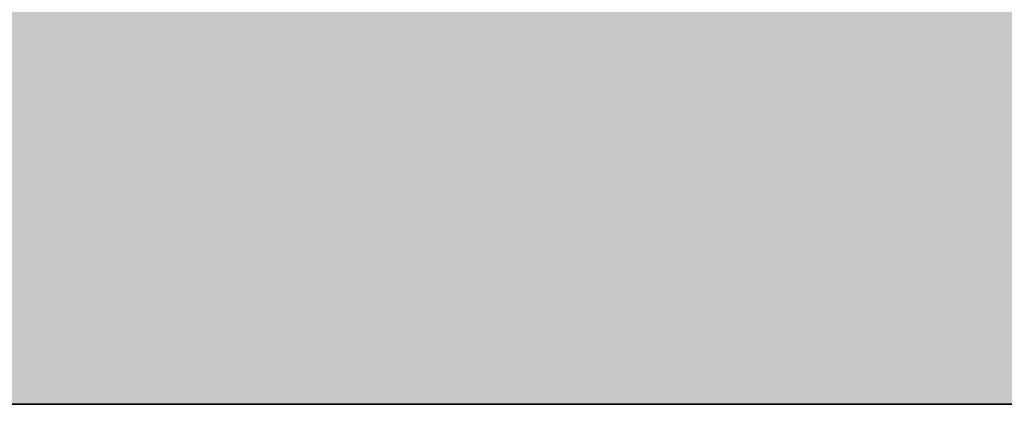
# Model space of a CAD drawing. Units: inches. Extents: x 2083 to 3317, y 1141 to 2115.
# Tile 145 of 256: x 3126.89136 to 3126.92826, y 1263.26136 to 1263.27577. Entities that reach past the tile are written whole.
import ezdxf

# ---------------------------------------------------------------- set-up
doc = ezdxf.new("R2010")
doc.units = ezdxf.units.IN
doc.layers.add('A-ANNO-DIMS', color=2, linetype='Continuous', lineweight=18)
doc.layers.add('A-WALL', color=7, linetype='Continuous', lineweight=35)
doc.layers.add('A-WALL-PATT', color=251, linetype='Continuous', lineweight=13, true_color=0x636466)
doc.styles.get("Standard").update_dxf_attribs({"font": 'arial.ttf'})
doc.dimstyles.new('ISO-25', dxfattribs={"dimtxt": 12, "dimasz": 12, "dimexe": 1.25, "dimexo": 0.625, "dimtad": 1, "dimlunit": 3, "dimtxsty": 'Standard', "dimcen": 2.5, "dimadec": 0, "dimazin": 0, "dimtfac": 1, "dimtmove": 0, "dimatfit": 3, "dimfxl": 1, "dimarcsym": 0})

# ---------------------------------------------------------------- blocks, each defined once
blk = doc.blocks.new('*D10')
at = {"layer": 'A-ANNO-DIMS', "color": 0, "lineweight": -2, "transparency": 16777216}
for p, q in [((2862.959783, 1262.63636), (2862.959783, 1201.38445)), ((3126.959783, 1262.63636), (3126.959783, 1201.38445)), ((2874.959783, 1202.63445), (3114.959783, 1202.63445))]:
    blk.add_line(p, q, dxfattribs=at)
at = {"layer": 'A-ANNO-DIMS', "color": 0, "transparency": 16777216}
for points in [[(2874.959783, 1204.63445), (2874.959783, 1200.63445), (2862.959783, 1202.63445)], [(3114.959783, 1204.63445), (3114.959783, 1200.63445), (3126.959783, 1202.63445)]]:
    blk.add_solid(points, dxfattribs=at)
at = {"layer": 'Defpoints', "color": 0, "transparency": 16777216}
for p in [(2862.959783, 1263.26136), (3126.959783, 1263.26136), (3126.959783, 1202.63445)]:
    blk.add_point(p, dxfattribs=at)
at = {"layer": 'A-ANNO-DIMS', "color": 0, "transparency": 16777216, "insert": (2994.959783, 1209.284006), "char_height": 12, "attachment_point": 5}
blk.add_mtext("22'", dxfattribs=at)
blk = doc.blocks.new('*D26')
at = {"layer": 'A-ANNO-DIMS', "color": 0, "lineweight": -2, "transparency": 16777216}
for p, q in [((3088.985844, 1274.915092), (3088.985844, 1270.951963)), ((3111.240037, 1274.915092), (3111.240037, 1270.951963)), ((3076.985844, 1272.201963), (2840.262447, 1272.201963)), ((3111.240037, 1272.201963), (3088.985844, 1272.201963)), ((3123.240037, 1272.201963), (3135.240037, 1272.201963))]:
    blk.add_line(p, q, dxfattribs=at)
at = {"layer": 'A-ANNO-DIMS', "color": 0, "transparency": 16777216}
for points in [[(3076.985844, 1274.201963), (3076.985844, 1270.201963), (3088.985844, 1272.201963)], [(3123.240037, 1274.201963), (3123.240037, 1270.201963), (3111.240037, 1272.201963)]]:
    blk.add_solid(points, dxfattribs=at)
at = {"layer": 'Defpoints', "color": 0, "transparency": 16777216}
for p in [(3088.985844, 1275.540092), (3111.240037, 1275.540092), (3088.985844, 1272.201963)]:
    blk.add_point(p, dxfattribs=at)
at = {"layer": 'A-ANNO-DIMS', "color": 0, "transparency": 16777216, "insert": (2952.624146, 1279.031602), "char_height": 12, "attachment_point": 5}
blk.add_mtext('NIGHTSTAND 1\'-10 1/2" TYP.', dxfattribs=at)
blk = doc.blocks.new('*D27')
at = {"layer": 'A-ANNO-DIMS', "color": 0, "lineweight": -2, "transparency": 16777216}
for p, q in [((3114.578165, 1309.794285), (3114.578165, 1321.794285)), ((3111.865037, 1297.794285), (3115.828165, 1297.794285)), ((3114.578165, 1297.794285), (3114.578165, 1275.540092)), ((3111.865037, 1275.540092), (3115.828165, 1275.540092)), ((3114.578165, 1263.540092), (3114.578165, 1140.988591))]:
    blk.add_line(p, q, dxfattribs=at)
at = {"layer": 'A-ANNO-DIMS', "color": 0, "transparency": 16777216}
for points in [[(3112.578165, 1309.794285), (3116.578165, 1309.794285), (3114.578165, 1297.794285)], [(3112.578165, 1263.540092), (3116.578165, 1263.540092), (3114.578165, 1275.540092)]]:
    blk.add_solid(points, dxfattribs=at)
at = {"layer": 'Defpoints', "color": 0, "transparency": 16777216}
for p in [(3111.240037, 1297.794285), (3111.240037, 1275.540092), (3114.578165, 1275.540092)]:
    blk.add_point(p, dxfattribs=at)
at = {"layer": 'A-ANNO-DIMS', "color": 0, "transparency": 16777216, "insert": (3107.748527, 1196.264342), "char_height": 12, "attachment_point": 5, "rotation": 90}
blk.add_mtext('1\'-10 1/2" TYP.', dxfattribs=at)

msp = doc.modelspace()

# ---------------------------------------------------------------- hatches: boundary and pattern name
at = {"layer": 'A-WALL-PATT'}
h = msp.add_hatch(color=256, dxfattribs=at)
h.dxf.hatch_style = 1
h.paths.add_polyline_path([(3126.959783, 2020.76136), (2748.959783, 2020.76136), (2604.959783, 2020.76136), (2226.959783, 2020.76136), (2226.959783, 1702.76136), (2466.959783, 1702.76136), (2466.959783, 1582.76136), (2418.959783, 1582.76136), (2418.959783, 1477.76136), (2226.959783, 1477.76136), (2226.959783, 1263.26136), (2544.959783, 1263.26136), (2544.959783, 1411.76136), (2604.959783, 1411.76136), (2685.959783, 1411.76136), (2685.959783, 1420.76136), (2604.959783, 1420.76136), (2604.959783, 1573.76136), (2604.959783, 1702.76136), (2604.959783, 2011.76136), (2748.959783, 2011.76136), (2748.959783, 1702.76136), (2862.959783, 1702.76136), (2862.959783, 1621.76136), (2871.959783, 1621.76136), (2871.959783, 1702.76136), (2883.959783, 1702.76136), (2883.959783, 1706.939459, -0.026459), (2883.959783, 1711.76136), (2757.959783, 1711.76136), (2757.959783, 1807.76136), (2787.959783, 1807.76136), (2787.959783, 1812.26136), (2757.959783, 1812.26136), (2757.959783, 2011.76136), (2877.959783, 2011.76136), (2877.959783, 1812.26136), (2847.959783, 1812.26136), (2847.959783, 1807.76136), (2889.835742, 1807.76136), (2889.835742, 1812.26136), (2882.459783, 1812.26136), (2882.459783, 2011.76136), (3117.959783, 2011.76136), (3117.959783, 1812.26136), (2937.835742, 1812.26136), (2937.835742, 1807.76136), (2995.709783, 1807.76136), (2995.709783, 1796.117666), (3000.209783, 1796.117666), (3000.209783, 1807.76136), (3117.959783, 1807.76136), (3117.959783, 1711.76136), (3000.209783, 1711.76136), (3000.209783, 1760.117666), (2998.572705, 1760.117666, -0.020711), (2995.709783, 1760.117666), (2995.709783, 1711.76136), (2931.959783, 1711.76136), (2931.959783, 1702.76136), (3126.959783, 1702.76136)])
h.paths.add_polyline_path([(2471.459783, 2011.76136), (2471.459783, 1810.01136), (2462.716936, 1810.01136), (2462.716936, 1805.51136), (2505.959783, 1805.51136), (2505.959783, 1810.01136), (2475.959783, 1810.01136), (2475.959783, 2011.76136), (2595.959783, 2011.76136), (2595.959783, 1810.01136), (2565.959783, 1810.01136), (2565.959783, 1805.51136), (2595.959783, 1805.51136), (2595.959783, 1711.76136), (2235.959783, 1711.76136), (2235.959783, 1805.51136), (2353.709783, 1805.51136), (2353.709783, 1796.054162), (2358.209783, 1796.054162), (2358.209783, 1805.51136), (2414.716936, 1805.51136), (2414.716936, 1810.01136), (2235.959783, 1810.01136), (2235.959783, 2011.76136)], flags=16)
h.paths.add_polyline_path([(2270.204734, 1994.610008), (2270.204734, 1970.610008), (2246.204734, 1970.610008), (2246.204734, 1994.610008)], flags=0)
edge = h.paths.add_edge_path(flags=0)
edge.add_ellipse((2332.027391, 1899.798176), major_axis=(-3.042994, 3.042994), ratio=0.16825245, start_angle=-161.332166, end_angle=-156.307114, ccw=False)
edge.add_ellipse((2333.082037, 1898.74353), major_axis=(-1.054646, 1.054646), ratio=0.4535321, start_angle=-123.371019, end_angle=-94.159107)
edge = h.paths.add_edge_path(flags=0)
edge.add_ellipse((2332.027391, 1968.87629), major_axis=(3.042994, 3.042994), ratio=0.16825245, start_angle=18.667834, end_angle=23.692886)
edge.add_spline(control_points=[(2332.925596, 1970.691105), (2332.226768, 1970.3361), (2330.893709, 1969.658905), (2328.41308, 1970.932138), (2327.203934, 1967.748712), (2324.709596, 1969.955589), (2322.532822, 1967.012354), (2320.012846, 1971.295812), (2317.680308, 1968.157845), (2316.040526, 1967.102047), (2315.426904, 1966.809602)], knot_values=[0, 0, 0, 0, 2.267059, 4.324559, 6.685584, 8.878641, 11.121502, 14.300359, 17.755284, 19.732645, 19.732645, 19.732645, 19.732645], degree=3, periodic=0)
edge.add_ellipse((2332.027391, 1968.87629), major_axis=(3.042994, 3.042994), ratio=0.16825245, start_angle=18.667834, end_angle=23.692886, ccw=False)
edge.add_ellipse((2333.082037, 1969.930936), major_axis=(1.054646, 1.054646), ratio=0.4535321, start_angle=56.628981, end_angle=85.840893, ccw=False)
edge = h.paths.add_edge_path(flags=0)
edge.add_spline(control_points=[(2296.428287, 1967.987908), (2293.627804, 1965.336314), (2287.703624, 1959.727094), (2299.74386, 1949.995699), (2294.532591, 1935.668528), (2290.573228, 1920.603512), (2293.394124, 1909.973691), (2296.185407, 1904.966543)], knot_values=[0.099185, 0.099185, 0.099185, 0.099185, 0.345301, 0.619822, 0.982653, 1.386093, 1.810555, 1.810555, 1.810555, 1.810555], degree=3, periodic=0)
edge.add_spline(control_points=[(2296.185407, 1904.966543), (2297.383582, 1902.6193), (2298.000969, 1901.949312), (2298.55297, 1901.468155)], knot_values=[0.006246, 0.006246, 0.006246, 0.006246, 0.055476, 0.055476, 0.055476, 0.055476], degree=3, periodic=0)
edge.add_spline(control_points=[(2298.55297, 1901.468155), (2297.258612, 1900.923224), (2295.225294, 1900.232126), (2293.060229, 1900.614205), (2292.101423, 1900.788415), (2292.089578, 1900.790568)], knot_values=[0.312835, 0.312835, 0.312835, 0.312835, 0.40178, 0.474987, 0.475903, 0.475903, 0.475903, 0.475903], degree=3, periodic=0)
edge.add_arc((2292.793646, 1904.664109), 3.937008, 215.420897, 259.698179, ccw=False)
edge.add_spline(control_points=[(2289.585314, 1902.382304), (2289.476652, 1902.535087), (2289.36848, 1902.688035), (2289.260865, 1902.84117)], knot_values=[0.102872, 0.102872, 0.102872, 0.102872, 0.116896, 0.116896, 0.116896, 0.116896], degree=3, periodic=0)
edge.add_spline(control_points=[(2289.260865, 1902.84117), (2288.686604, 1902.550192), (2287.640048, 1902.019902), (2285.881337, 1901.873954), (2283.852972, 1901.504352), (2281.719987, 1899.710538), (2278.466991, 1899.492942), (2276.157136, 1901.883202), (2272.258953, 1899.804071), (2267.777605, 1901.843183), (2262.243882, 1900.184033), (2257.414927, 1901.782061), (2254.318374, 1900.72612), (2253.178285, 1900.337343)], knot_values=[0, 0, 0, 0, 1.907977, 3.477176, 5.261074, 7.972851, 11.680248, 13.717921, 16.939592, 22.789562, 27.502503, 33.595215, 37.145618, 37.145618, 37.145618, 37.145618], degree=3, periodic=0)
edge.add_line((2253.178285, 1900.337343), (2250.24424, 1902.84117))
edge.add_line((2250.24424, 1902.84117), (2250.24424, 1965.833296))
edge.add_line((2250.24424, 1965.833296), (2253.178285, 1968.337123))
edge.add_spline(control_points=[(2253.178285, 1968.337123), (2254.318374, 1967.948346), (2257.414927, 1966.892405), (2262.243882, 1968.490433), (2267.777605, 1966.831283), (2271.52673, 1968.537217), (2273.875914, 1967.828289), (2274.206701, 1967.727642)], knot_values=[0, 0, 0, 0, 0.09018, 0.244935, 0.364644, 0.513233, 0.537855, 0.537855, 0.537855, 0.537855], degree=3, periodic=0)
edge.add_arc((2274.352887, 1963.793349), 3.937008, 72.051134, 92.127949, ccw=False)
edge.add_arc((2281.296933, 1985.230003), 18.596298, 252.0511336, 288.5657217)
edge.add_arc((2292.316717, 1956.02888), 12.646081, 71.0267879, 113.7782184, ccw=False)
edge = h.paths.add_edge_path(flags=0)
edge.add_spline(control_points=[(2274.899415, 1951.856195), (2275.066156, 1951.616592), (2275.232687, 1951.376588), (2275.397987, 1951.135855)], knot_values=[1.409916, 1.409916, 1.409916, 1.409916, 1.43159, 1.43159, 1.43159, 1.43159], degree=3, periodic=0)
edge.add_spline(control_points=[(2275.397987, 1951.135855), (2275.792106, 1950.561885), (2276.179231, 1949.983774), (2276.545546, 1949.397103)], knot_values=[1.358238, 1.358238, 1.358238, 1.358238, 1.409916, 1.409916, 1.409916, 1.409916], degree=3, periodic=0)
edge.add_line((2276.545546, 1949.397103), (2277.437289, 1947.862185))
edge.add_spline(control_points=[(2277.437289, 1947.862185), (2276.303834, 1945.673115), (2274.639698, 1942.426882), (2274.631615, 1938.0939), (2272.799124, 1930.85155), (2274.356426, 1943.897046), (2275.947681, 1947.923356), (2276.545546, 1949.397103)], knot_values=[0.005632, 0.005632, 0.005632, 0.005632, 0.186014, 0.266002, 0.357087, 0.59639, 0.739732, 0.739732, 0.739732, 0.739732], degree=3, periodic=0)
edge.add_spline(control_points=[(2276.545546, 1949.397103), (2276.179231, 1949.983774), (2275.792106, 1950.561885), (2275.397987, 1951.135855)], knot_values=[1.358238, 1.358238, 1.358238, 1.358238, 1.409916, 1.409916, 1.409916, 1.409916], degree=3, periodic=0)
edge.add_spline(control_points=[(2275.397987, 1951.135855), (2274.9425, 1950.080452), (2274.20776, 1948.025272), (2273.934602, 1944.851477), (2272.468534, 1937.627489), (2273.466216, 1945.696466), (2274.700615, 1951.059472), (2274.899415, 1951.856195)], knot_values=[0.104364, 0.104364, 0.104364, 0.104364, 0.189636, 0.269624, 0.36071, 0.600013, 0.644622, 0.644622, 0.644622, 0.644622], degree=3, periodic=0)
h.paths.add_polyline_path([(2269.167514, 1963.127573, -0.357527), (2268.170633, 1960.97637, -0.092561), (2268.170633, 1939.436325, -0.357527), (2269.167514, 1937.285122, -0.357527), (2267.01631, 1938.282002, -0.164785), (2254.685581, 1938.282002, -0.357527), (2252.534378, 1937.285122, -0.357527), (2253.531259, 1939.436325, -0.092561), (2253.531259, 1960.97637, -0.357527), (2252.534378, 1963.127573, -0.357527), (2254.685581, 1962.130692, -0.164785), (2267.01631, 1962.130692, -0.357527)], flags=0)
h.paths.add_polyline_path([(2248.874068, 1967.8018), (2248.874068, 1957.02771), (2249.457783, 1957.02771), (2249.457783, 1911.646756), (2248.874068, 1911.646756), (2248.874068, 1900.872666), (2246.511863, 1900.872666, 0.197327), (2244.149658, 1902.456873), (2244.149658, 1966.217592, 0.197327), (2246.511863, 1967.8018)], flags=0)
h.paths.add_polyline_path([(2269.167514, 1931.389344, -0.357527), (2268.170633, 1929.238141, -0.092561), (2268.170633, 1907.698096, -0.357527), (2269.167514, 1905.546893, -0.357527), (2267.01631, 1906.543774, -0.164785), (2254.685581, 1906.543774, -0.357527), (2252.534378, 1905.546893, -0.357527), (2253.531259, 1907.698096, -0.092561), (2253.531259, 1929.238141, -0.357527), (2252.534378, 1931.389344, -0.357527), (2254.685581, 1930.392463, -0.164785), (2267.01631, 1930.392463, -0.357527)], flags=0)
edge = h.paths.add_edge_path(flags=0)
edge.add_spline(control_points=[(2276.196858, 1906.723702), (2276.168144, 1909.028928), (2276.114049, 1913.371852), (2270.598417, 1924.924978), (2273.905175, 1919.012779), (2275.921711, 1916.262063), (2275.47457, 1912.402149), (2277.257874, 1910.380621), (2276.696044, 1908.225036), (2276.646218, 1906.813023), (2276.617825, 1906.008407)], knot_values=[0, 0, 0, 0, 8.61026, 16.221274, 18.843057, 23.804898, 27.440828, 29.356102, 31.203478, 33.650687, 33.650687, 33.650687, 33.650687], degree=3, periodic=0)
edge.add_spline(control_points=[(2276.617825, 1906.008407), (2276.623313, 1905.624144), (2276.497738, 1904.628661), (2275.441779, 1903.854725), (2274.937314, 1903.08045), (2274.85908, 1902.84117)], knot_values=[0.156488, 0.156488, 0.156488, 0.156488, 0.184398, 0.231376, 0.250598, 0.250598, 0.250598, 0.250598], degree=3, periodic=0)
edge.add_line((2274.85908, 1902.84117), (2276.50598, 1902.84117))
edge.add_spline(control_points=[(2276.50598, 1902.84117), (2276.788308, 1903.08494), (2277.665071, 1904.125196), (2278.249538, 1904.340738), (2277.653872, 1908.527387), (2278.15567, 1906.227808), (2278.100464, 1905.285948), (2278.846675, 1904.069005), (2277.856785, 1903.414948), (2277.874191, 1902.99105), (2277.903562, 1902.84117)], knot_values=[0.059574, 0.059574, 0.059574, 0.059574, 0.080753, 0.103741, 0.16972, 0.176036, 0.207137, 0.240474, 0.262341, 0.27366, 0.27366, 0.27366, 0.27366], degree=3, periodic=0)
edge.add_line((2277.903562, 1902.84117), (2280.029825, 1902.84117))
edge.add_spline(control_points=[(2280.029825, 1902.84117), (2279.888221, 1903.088398), (2279.499257, 1903.981551), (2280.152284, 1905.939349), (2278.103615, 1909.657757), (2279.762395, 1907.185285), (2280.3279, 1904.874861), (2280.485109, 1903.48959), (2281.463269, 1903.249432), (2281.758343, 1902.936497), (2281.834036, 1902.84117)], knot_values=[0.013856, 0.013856, 0.013856, 0.013856, 0.034874, 0.088867, 0.107879, 0.126738, 0.158714, 0.193757, 0.217487, 0.226722, 0.226722, 0.226722, 0.226722], degree=3, periodic=0)
edge.add_spline(control_points=[(2281.834036, 1902.84117), (2281.787535, 1902.826703), (2281.647022, 1902.782988), (2281.395527, 1902.85949), (2281.088077, 1902.985242), (2280.720683, 1903.060902), (2280.333451, 1903.025726), (2280.124767, 1902.898879), (2280.029825, 1902.84117)], knot_values=[0, 0, 0, 0, 0.14413, 0.435517, 0.749276, 1.153046, 1.548371, 1.878348, 1.878348, 1.878348, 1.878348], degree=3, periodic=0)
edge.add_line((2280.029825, 1902.84117), (2277.903562, 1902.84117))
edge.add_spline(control_points=[(2277.903562, 1902.84117), (2277.892855, 1902.795855), (2277.865396, 1902.679637), (2277.607479, 1902.687483), (2277.27405, 1902.8007), (2276.837921, 1902.619775), (2276.583807, 1902.789261), (2276.50598, 1902.84117)], knot_values=[0, 0, 0, 0, 0.127189, 0.326199, 0.628009, 1.24357, 1.515331, 1.515331, 1.515331, 1.515331], degree=3, periodic=0)
edge.add_line((2276.50598, 1902.84117), (2274.85908, 1902.84117))
edge.add_spline(control_points=[(2274.85908, 1902.84117), (2274.814437, 1902.898587), (2274.72513, 1903.013446), (2274.493477, 1903.118968), (2274.244285, 1902.960539), (2273.937121, 1903.184942), (2273.614039, 1902.983143), (2273.408316, 1902.883045), (2273.322254, 1902.84117)], knot_values=[0, 0, 0, 0, 0.21843, 0.436957, 0.687977, 0.990379, 1.398396, 1.69185, 1.69185, 1.69185, 1.69185], degree=3, periodic=0)
edge.add_spline(control_points=[(2273.322254, 1902.84117), (2273.61674, 1903.445692), (2274.273998, 1904.538253), (2276.027239, 1904.573702), (2276.206963, 1906.583637), (2276.196858, 1906.723702)], knot_values=[0.012227, 0.012227, 0.012227, 0.012227, 0.059472, 0.106218, 0.134458, 0.134458, 0.134458, 0.134458], degree=3, periodic=0)
h.paths.add_polyline_path([(2270.776054, 1897.789828), (2270.776054, 1873.789828), (2246.776054, 1873.789828), (2246.776054, 1897.789828)], flags=0)
h.paths.add_polyline_path([(2353.709783, 1760.005059), (2353.709783, 1760.054162), (2358.209783, 1760.054162, -0.033729)], flags=0)
h.paths.add_polyline_path([(2321.819119, 1737.529186), (2341.995327, 1737.529186, -0.414214), (2343.203273, 1736.321241), (2343.203273, 1721.020596, -0.414214), (2341.995327, 1719.812651), (2321.819119, 1719.812651, -0.414214), (2320.611173, 1721.020596), (2320.611173, 1736.321241, -0.414214)], flags=0)
h.paths.add_polyline_path([(2324.23501, 1736.321241), (2339.579436, 1736.321241, -0.414214), (2341.995327, 1733.905349), (2341.995327, 1725.44973, -0.414214), (2339.579436, 1723.033839), (2333.680588, 1723.033839), (2333.845317, 1722.045467, -0.870646), (2335.425399, 1721.825893, -0.767327), (2333.922694, 1721.423245), (2331.291024, 1721.423245, -0.767327), (2329.788319, 1721.825893, -0.870646), (2331.368401, 1722.045467), (2331.53313, 1723.033839), (2324.23501, 1723.033839, -0.414214), (2321.819119, 1725.44973), (2321.819119, 1733.905349, -0.414214)], flags=0)
h.paths.add_polyline_path([(2570.483789, 1928.615444), (2589.683789, 1928.615444), (2590.168829, 1928.615444), (2590.168829, 1904.993397), (2570.483789, 1904.993397)], flags=0)
h.paths.add_polyline_path([(2574.447324, 1927.263822, -1), (2572.828836, 1927.263822, -1)], flags=0)
h.paths.add_polyline_path([(2573.089867, 1926.940877), (2573.925032, 1927.776042), (2574.147743, 1927.553332), (2573.312577, 1926.718166)], flags=0)
h.paths.add_polyline_path([(2578.779065, 1919.729618, -1), (2571.591663, 1919.729618, -1)], flags=0)
h.paths.add_polyline_path([(2578.385364, 1919.729618, -1), (2571.985364, 1919.729618, -1)], flags=0)
h.paths.add_polyline_path([(2331.595764, 1729.476216, -1), (2333.617954, 1729.476216, -1)], flags=0)
h.paths.add_polyline_path([(2578.034228, 1927.263822, -1), (2576.41574, 1927.263822, -1)], flags=0)
h.paths.add_polyline_path([(2576.688851, 1927.531089), (2576.911562, 1927.753799), (2577.746728, 1926.918634), (2577.524017, 1926.695923)], flags=0)
h.paths.add_polyline_path([(2578.139065, 1909.859539, -1), (2572.231663, 1909.859539, -1)], flags=0)
h.paths.add_polyline_path([(2577.745364, 1909.859539, -1), (2572.625364, 1909.859539, -1)], flags=0)
h.paths.add_polyline_path([(2583.797718, 1927.263822, -1), (2582.179229, 1927.263822, -1)], flags=0)
h.paths.add_polyline_path([(2582.718649, 1927.753799), (2583.553814, 1926.918634), (2583.331103, 1926.695923), (2582.495938, 1927.531089)], flags=0)
h.paths.add_polyline_path([(2582.495938, 1927.531089), (2582.718649, 1927.753799), (2583.553814, 1926.918634), (2583.331103, 1926.695923)], flags=0)
h.paths.add_polyline_path([(2587.739065, 1920.529618, -1), (2581.831663, 1920.529618, -1)], flags=0)
h.paths.add_polyline_path([(2587.345364, 1920.529618, -1), (2582.225364, 1920.529618, -1)], flags=0)
h.paths.add_polyline_path([(2587.384622, 1927.263822, -1), (2585.766133, 1927.263822, -1)], flags=0)
h.paths.add_polyline_path([(2586.081993, 1926.980247), (2586.917158, 1927.815412), (2587.139869, 1927.592702), (2586.304703, 1926.757536)], flags=0)
h.paths.add_polyline_path([(2588.379065, 1910.659539, -1), (2581.191663, 1910.659539, -1)], flags=0)
h.paths.add_polyline_path([(2587.985364, 1910.659539, -1), (2581.585364, 1910.659539, -1)], flags=0)
h.paths.add_polyline_path([(2417.167729, 1729.477895), (2437.343937, 1729.477895, -0.414214), (2438.551883, 1728.26995), (2438.551883, 1712.969306, -0.414214), (2437.343937, 1711.76136), (2417.167729, 1711.76136, -0.414214), (2415.959783, 1712.969306), (2415.959783, 1728.26995, -0.414214)], flags=0)
h.paths.add_polyline_path([(2419.58362, 1728.26995), (2434.928046, 1728.26995, -0.414214), (2437.343937, 1725.854059), (2437.343937, 1717.39844, -0.414214), (2434.928046, 1714.982548), (2429.029199, 1714.982548), (2429.193927, 1713.994176, -0.870646), (2430.774009, 1713.774603, -0.767327), (2429.271304, 1713.371954), (2426.639634, 1713.371954, -0.767327), (2425.136929, 1713.774603, -0.870646), (2426.717011, 1713.994176), (2426.88174, 1714.982548), (2419.58362, 1714.982548, -0.414214), (2417.167729, 1717.39844), (2417.167729, 1725.854059, -0.414214)], flags=0)
h.paths.add_polyline_path([(2419.58362, 1728.26995), (2434.928046, 1728.26995, -0.414214), (2437.343937, 1725.854059), (2437.343937, 1717.39844, -0.414214), (2434.928046, 1714.982548), (2429.029199, 1714.982548), (2428.358118, 1719.009034), (2427.552821, 1719.009034), (2426.88174, 1714.982548), (2419.58362, 1714.982548, -0.414214), (2417.167729, 1717.39844), (2417.167729, 1725.854059, -0.414214)], flags=0)
h.paths.add_polyline_path([(2426.944374, 1721.424925, -1), (2428.966564, 1721.424925, -1)], flags=0)
h.paths.add_polyline_path([(2475.959783, 1702.76136), (2595.959783, 1702.76136), (2595.959783, 1582.76136), (2475.959783, 1582.76136)], flags=16)
h.paths.add_polyline_path([(2427.959783, 1573.76136), (2595.959783, 1573.76136), (2595.959783, 1468.76136), (2595.959783, 1420.76136), (2384.459783, 1420.76136), (2384.459783, 1468.76136), (2427.959783, 1468.76136)], flags=16)
h.paths.add_polyline_path([(2379.959783, 1468.76136), (2379.959783, 1420.76136), (2235.959783, 1420.76136), (2235.959783, 1468.76136)], flags=16)
h.paths.add_polyline_path([(2317.815996, 1466.695767), (2337.992205, 1466.695767, -0.414214), (2339.20015, 1465.487821), (2339.20015, 1450.187177, -0.414214), (2337.992205, 1448.979232), (2317.815996, 1448.979232, -0.414214), (2316.608051, 1450.187177), (2316.608051, 1465.487821, -0.414214)], flags=0)
h.paths.add_polyline_path([(2320.231887, 1465.487821), (2335.576313, 1465.487821, -0.414214), (2337.992205, 1463.07193), (2337.992205, 1454.616311, -0.414214), (2335.576313, 1452.20042), (2329.677466, 1452.20042), (2329.842195, 1451.212047, -0.870646), (2331.422276, 1450.992474, -0.767327), (2329.919571, 1450.589826), (2327.287902, 1450.589826, -0.767327), (2325.785197, 1450.992474, -0.870646), (2327.365278, 1451.212047), (2327.530007, 1452.20042), (2320.231887, 1452.20042, -0.414214), (2317.815996, 1454.616311), (2317.815996, 1463.07193, -0.414214)], flags=0)
h.paths.add_polyline_path([(2320.231887, 1465.487821), (2335.576313, 1465.487821, -0.414214), (2337.992205, 1463.07193), (2337.992205, 1454.616311, -0.414214), (2335.576313, 1452.20042), (2329.677466, 1452.20042), (2329.006385, 1456.226905), (2328.201088, 1456.226905), (2327.530007, 1452.20042), (2320.231887, 1452.20042, -0.414214), (2317.815996, 1454.616311), (2317.815996, 1463.07193, -0.414214)], flags=0)
h.paths.add_polyline_path([(2327.592641, 1458.642796, -1), (2329.614832, 1458.642796, -1)], flags=0)
h.paths.add_polyline_path([(2244.411744, 1433.340453), (2241.920945, 1433.340453, -0.414214), (2240.017856, 1435.243542), (2240.017856, 1440.952808, -0.414211), (2241.920925, 1442.855897), (2244.411744, 1442.855897, -1.976472)], flags=0)
h.paths.add_polyline_path([(2245.356888, 1434.397536, -0.414214), (2245.356888, 1441.798814, -2.144098)], flags=0)
h.paths.add_polyline_path([(2535.959783, 1416.26136), (2535.959783, 1272.26136), (2235.959783, 1272.26136), (2235.959783, 1416.26136)], flags=16)
h.paths.add_polyline_path([(2260.119561, 1384.292841), (2260.119561, 1362.038649), (2237.865369, 1362.038649), (2237.865369, 1384.292841)], flags=0)
edge = h.paths.add_edge_path(flags=0)
edge.add_line((2318.251847, 1362.093298), (2318.145797, 1362.000973))
edge.add_ellipse((2317.445116, 1360.431044), major_axis=(2.82164, 2.82164), ratio=0.16825245, start_angle=18.667834, end_angle=20.948127, ccw=False)
edge.add_ellipse((2318.423045, 1361.408974), major_axis=(0.977929, 0.977929), ratio=0.4535321, start_angle=56.628981, end_angle=70.226201, ccw=False)
edge = h.paths.add_edge_path(flags=0)
edge.add_line((2319.10737, 1295.571078), (2319.015044, 1295.677128))
edge.add_ellipse((2317.445116, 1296.377809), major_axis=(-2.82164, 2.82164), ratio=0.16825245, start_angle=-161.332166, end_angle=-159.051873, ccw=False)
edge.add_ellipse((2318.423045, 1295.39988), major_axis=(-0.977929, 0.977929), ratio=0.4535321, start_angle=-123.371019, end_angle=-109.773799)
edge = h.paths.add_edge_path(flags=0)
edge.add_spline(control_points=[(2284.210349, 1301.170219), (2284.580688, 1300.444719), (2284.891189, 1299.892024), (2285.159553, 1299.461018)], knot_values=[0.039066, 0.039066, 0.039066, 0.039066, 0.055476, 0.055476, 0.055476, 0.055476], degree=3, periodic=0)
edge.add_line((2285.159553, 1299.461018), (2284.210349, 1301.170219))
edge = h.paths.add_edge_path(flags=0)
edge.add_line((2280.412458, 1297.298013), (2283.369991, 1297.036122))
edge.add_line((2283.369991, 1297.036122), (2286.40569, 1297.92631))
edge.add_spline(control_points=[(2286.40569, 1297.92631), (2285.305487, 1297.463119), (2284.344777, 1297.129151), (2283.369991, 1297.036122)], knot_values=[0.394369, 0.394369, 0.394369, 0.394369, 0.475903, 0.475903, 0.475903, 0.475903], degree=3, periodic=0)
edge.add_spline(control_points=[(2283.369991, 1297.036122), (2283.28139, 1297.027666), (2282.316289, 1296.957336), (2281.312502, 1297.134479), (2280.423441, 1297.296016), (2280.412458, 1297.298013)], knot_values=[0.312835, 0.312835, 0.312835, 0.312835, 0.320246, 0.393453, 0.394369, 0.394369, 0.394369, 0.394369], degree=3, periodic=0)
edge = h.paths.add_edge_path(flags=0)
edge.add_line((2284.435561, 1359.607285), (2280.446291, 1355.328047))
edge.add_line((2280.446291, 1355.328047), (2279.579987, 1351.017754))
edge.add_line((2279.579987, 1351.017754), (2282.412974, 1346.580433))
edge.add_spline(control_points=[(2282.412974, 1346.580433), (2283.153331, 1345.589236), (2284.252896, 1344.028897), (2284.801037, 1342.387167), (2284.935162, 1341.805544)], knot_values=[1.240098, 1.240098, 1.240098, 1.240098, 1.332892, 1.382712, 1.382712, 1.382712, 1.382712], degree=3, periodic=0)
edge.add_spline(control_points=[(2284.935162, 1341.805544), (2285.319108, 1340.1406), (2285.233029, 1338.409204), (2284.909938, 1336.654122)], knot_values=[1.097484, 1.097484, 1.097484, 1.097484, 1.240098, 1.240098, 1.240098, 1.240098], degree=3, periodic=0)
edge.add_spline(control_points=[(2284.909938, 1336.654122), (2284.586848, 1334.89904), (2284.026745, 1333.120272), (2283.462644, 1331.360585)], knot_values=[0.95487, 0.95487, 0.95487, 0.95487, 1.097484, 1.097484, 1.097484, 1.097484], degree=3, periodic=0)
edge.add_line((2283.462644, 1331.360585), (2281.890376, 1326.153357))
edge.add_line((2281.890376, 1326.153357), (2280.756259, 1321.056089))
edge.add_line((2280.756259, 1321.056089), (2280.299205, 1316.001977))
edge.add_line((2280.299205, 1316.001977), (2280.715933, 1310.950068))
edge.add_line((2280.715933, 1310.950068), (2282.028094, 1305.972137))
edge.add_line((2282.028094, 1305.972137), (2284.210349, 1301.170219))
edge.add_spline(control_points=[(2284.210349, 1301.170219), (2283.340731, 1302.730185), (2282.611904, 1304.336493), (2282.028094, 1305.972137)], knot_values=[0.099185, 0.099185, 0.099185, 0.099185, 0.241799, 0.241799, 0.241799, 0.241799], degree=3, periodic=0)
edge.add_spline(control_points=[(2282.028094, 1305.972137), (2281.444283, 1307.60778), (2281.005489, 1309.272759), (2280.715933, 1310.950068)], knot_values=[0.241799, 0.241799, 0.241799, 0.241799, 0.384413, 0.384413, 0.384413, 0.384413], degree=3, periodic=0)
edge.add_spline(control_points=[(2280.715933, 1310.950068), (2280.433241, 1312.587613), (2280.289386, 1314.276959), (2280.298894, 1315.962032), (2280.299205, 1316.001977)], knot_values=[0.384413, 0.384413, 0.384413, 0.384413, 0.523647, 0.527028, 0.527028, 0.527028, 0.527028], degree=3, periodic=0)
edge.add_spline(control_points=[(2280.299205, 1316.001977), (2280.312326, 1317.686955), (2280.477871, 1319.367926), (2280.756259, 1321.056089)], knot_values=[0.527028, 0.527028, 0.527028, 0.527028, 0.669642, 0.669642, 0.669642, 0.669642], degree=3, periodic=0)
edge.add_spline(control_points=[(2280.756259, 1321.056089), (2281.034648, 1322.744252), (2281.42588, 1324.439608), (2281.890376, 1326.153357)], knot_values=[0.669642, 0.669642, 0.669642, 0.669642, 0.812256, 0.812256, 0.812256, 0.812256], degree=3, periodic=0)
edge.add_spline(control_points=[(2281.890376, 1326.153357), (2282.264383, 1327.533251), (2282.78787, 1329.26181), (2283.352751, 1331.01778), (2283.462644, 1331.360585)], knot_values=[0.812256, 0.812256, 0.812256, 0.812256, 0.927087, 0.95487, 0.95487, 0.95487, 0.95487], degree=3, periodic=0)
edge.add_line((2283.462644, 1331.360585), (2284.909938, 1336.654122))
edge.add_line((2284.909938, 1336.654122), (2284.935162, 1341.805544))
edge.add_line((2284.935162, 1341.805544), (2282.412974, 1346.580433))
edge.add_spline(control_points=[(2282.412974, 1346.580433), (2281.275127, 1348.103792), (2280.078447, 1349.570318), (2279.579987, 1351.017754)], knot_values=[1.382712, 1.382712, 1.382712, 1.382712, 1.525326, 1.525326, 1.525326, 1.525326], degree=3, periodic=0)
edge.add_spline(control_points=[(2279.579987, 1351.017754), (2279.443282, 1351.414721), (2279.136312, 1352.856922), (2279.73519, 1354.290385), (2280.446291, 1355.328047)], knot_values=[1.525326, 1.525326, 1.525326, 1.525326, 1.564439, 1.667941, 1.667941, 1.667941, 1.667941], degree=3, periodic=0)
edge.add_spline(control_points=[(2280.446291, 1355.328047), (2281.426113, 1356.757835), (2282.930837, 1358.18256), (2284.435561, 1359.607285)], knot_values=[1.667941, 1.667941, 1.667941, 1.667941, 1.810555, 1.810555, 1.810555, 1.810555], degree=3, periodic=0)
edge.add_arc((2280.623075, 1348.518181), 11.72618, 71.0267879, 113.7782184)
edge.add_arc((2270.404892, 1375.595156), 17.243567, 252.0511336, 288.5657217, ccw=False)
edge.add_arc((2263.965969, 1355.717847), 3.650622, 72.051134, 92.127949)
edge.add_arc((2263.965969, 1355.717847), 3.650622, 92.127949, 177.98513)
edge.add_spline(control_points=[(2260.317604, 1355.846199), (2260.260417, 1354.220668), (2260.551278, 1350.186547), (2262.999344, 1346.766251), (2264.472741, 1344.649024)], knot_values=[1.43159, 1.43159, 1.43159, 1.43159, 1.564144, 1.770695, 1.770695, 1.770695, 1.770695], degree=3, periodic=0)
edge.add_line((2264.472741, 1344.649024), (2264.93559, 1343.98253))
edge.add_spline(control_points=[(2263.801044, 1340.248105), (2263.843238, 1340.514088), (2264.067244, 1341.756465), (2264.512693, 1343.002453), (2264.935047, 1343.981083)], knot_values=[0.53657, 0.53657, 0.53657, 0.53657, 0.559349, 0.644622, 0.644622, 0.644622, 0.644622], degree=3, periodic=0)
edge.add_spline(control_points=[(2264.935047, 1343.981083), (2265.117771, 1343.714975), (2265.298875, 1343.447906), (2265.476756, 1343.179365)], knot_values=[1.384077, 1.384077, 1.384077, 1.384077, 1.409916, 1.409916, 1.409916, 1.409916], degree=3, periodic=0)
edge.add_spline(control_points=[(2265.476756, 1343.179365), (2265.654637, 1342.910823), (2265.829296, 1342.64081), (2265.99913, 1342.368812)], knot_values=[1.358238, 1.358238, 1.358238, 1.358238, 1.384077, 1.384077, 1.384077, 1.384077], degree=3, periodic=0)
edge.add_line((2265.99913, 1342.368812), (2266.826006, 1340.945547))
edge.add_spline(control_points=[(2266.826006, 1340.945547), (2268.894401, 1337.089691), (2271.398173, 1325.843001), (2270.516164, 1310.568557), (2275.919376, 1301.860609), (2277.789511, 1299.19945)], knot_values=[0.116896, 0.116896, 0.116896, 0.116896, 0.472987, 1.050969, 1.313793, 1.313793, 1.313793, 1.313793], degree=3, periodic=0)
edge.add_spline(control_points=[(2277.789511, 1299.19945), (2277.839405, 1299.128452), (2277.889428, 1299.057498), (2277.939572, 1298.986584)], knot_values=[0.109884, 0.109884, 0.109884, 0.109884, 0.116896, 0.116896, 0.116896, 0.116896], degree=3, periodic=0)
edge.add_line((2277.939572, 1298.986584), (2277.788849, 1299.199114))
edge.add_spline(control_points=[(2277.788849, 1299.199114), (2277.256582, 1298.929414), (2276.28635, 1298.437902), (2275.039352, 1298.334419), (2274.38333, 1298.238895), (2274.215254, 1298.209338)], knot_values=[33.12187, 33.12187, 33.12187, 33.12187, 35.029056, 36.598255, 37.144827, 37.144827, 37.144827, 37.144827], degree=3, periodic=0)
edge.add_line((2274.215254, 1298.209338), (2273.073147, 1297.892961))
edge.add_spline(control_points=[(2273.073147, 1297.892961), (2272.322936, 1297.579784), (2271.039151, 1296.510508), (2269.248395, 1296.226062), (2268.4231, 1296.374654)], knot_values=[26.532584, 26.532584, 26.532584, 26.532584, 29.198919, 31.839101, 31.839101, 31.839101, 31.839101], degree=3, periodic=0)
edge.add_line((2268.4231, 1296.374654), (2263.878501, 1297.457534))
edge.add_spline(control_points=[(2263.878501, 1297.457534), (2263.556077, 1297.359435), (2261.860306, 1296.838694), (2260.23878, 1297.282407), (2258.933454, 1297.516461)], knot_values=[15.919551, 15.919551, 15.919551, 15.919551, 16.939592, 21.226067, 21.226067, 21.226067, 21.226067], degree=3, periodic=0)
edge.add_line((2258.933454, 1297.516461), (2254.055233, 1297.32901))
edge.add_spline(control_points=[(2254.055233, 1297.32901), (2253.755525, 1297.295815), (2252.113683, 1297.165174), (2250.461869, 1297.544221), (2249.129686, 1297.667882)], knot_values=[5.306517, 5.306517, 5.306517, 5.306517, 6.276435, 10.613034, 10.613034, 10.613034, 10.613034], degree=3, periodic=0)
edge.add_line((2249.129686, 1297.667882), (2244.33165, 1296.877756))
edge.add_line((2244.33165, 1296.877756), (2241.611033, 1299.19945))
edge.add_line((2241.611033, 1299.19945), (2241.611033, 1357.609404))
edge.add_line((2241.611033, 1357.609404), (2244.33165, 1359.931097))
edge.add_line((2244.33165, 1359.931097), (2252.728823, 1359.542692))
edge.add_spline(control_points=[(2252.728823, 1359.542692), (2252.870939, 1359.54644), (2253.30574, 1359.548172), (2253.739845, 1359.514274), (2254.031742, 1359.482426)], knot_values=[0.233291, 0.233291, 0.233291, 0.233291, 0.244935, 0.268927, 0.268927, 0.268927, 0.268927], degree=3, periodic=0)
edge.add_line((2254.031742, 1359.482426), (2259.58719, 1359.41639))
edge.add_spline(control_points=[(2259.58719, 1359.41639), (2260.677068, 1359.628503), (2262.073197, 1359.897003), (2263.523692, 1359.459278), (2263.830417, 1359.365952)], knot_values=[0.422516, 0.422516, 0.422516, 0.422516, 0.513233, 0.537855, 0.537855, 0.537855, 0.537855], degree=3, periodic=0)
edge.add_arc((2263.965969, 1355.717847), 3.650622, 72.051134, 92.127949, ccw=False)
edge.add_arc((2270.404892, 1375.595156), 17.243567, 252.0511336, 288.5657217)
edge.add_arc((2280.623075, 1348.518181), 11.72618, 71.0267879, 113.7782184, ccw=False)
h.paths.add_polyline_path([(2240.34053, 1359.434715), (2240.34053, 1349.444353), (2240.881785, 1349.444353), (2240.881785, 1307.3645), (2240.34053, 1307.3645), (2240.34053, 1297.374138), (2238.150157, 1297.374138, 0.197327), (2235.959783, 1298.843108), (2235.959783, 1357.965746, 0.197327), (2238.150157, 1359.434715)], flags=0)
h.paths.add_polyline_path([(2259.15779, 1355.1005, -0.357527), (2258.233425, 1353.10578, -0.092561), (2258.233425, 1333.132601, -0.357527), (2259.15779, 1331.13788, -0.357527), (2257.16307, 1332.062246, -0.164785), (2245.729302, 1332.062246, -0.357527), (2243.734582, 1331.13788, -0.357527), (2244.658947, 1333.132601, -0.092561), (2244.658947, 1353.10578, -0.357527), (2243.734582, 1355.1005, -0.357527), (2245.729302, 1354.176135, -0.164785), (2257.16307, 1354.176135, -0.357527)], flags=0)
edge = h.paths.add_edge_path(flags=0)
edge.add_line((2265.99913, 1342.368812), (2266.826006, 1340.945547))
edge.add_line((2266.826006, 1340.945547), (2265.307557, 1337.814066))
edge.add_line((2265.307557, 1337.814066), (2264.358232, 1334.652939))
edge.add_line((2264.358232, 1334.652939), (2264.262012, 1333.799705))
edge.add_spline(control_points=[(2264.262012, 1333.799705), (2264.208357, 1333.187055), (2264.16206, 1332.365525), (2264.007144, 1331.413933), (2263.969049, 1331.201834)], knot_values=[0.464444, 0.464444, 0.464444, 0.464444, 0.516691, 0.531608, 0.531608, 0.531608, 0.531608], degree=3, periodic=0)
edge.add_spline(control_points=[(2263.969049, 1331.201834), (2263.774535, 1330.118873), (2263.42437, 1328.790839), (2263.25742, 1328.530652), (2263.234028, 1328.514612)], knot_values=[0.372682, 0.372682, 0.372682, 0.372682, 0.44885, 0.464444, 0.464444, 0.464444, 0.464444], degree=3, periodic=0)
edge.add_spline(control_points=[(2263.234028, 1328.514612), (2263.096382, 1328.420227), (2263.13117, 1329.301477), (2263.274953, 1330.615749)], knot_values=[0.280919, 0.280919, 0.280919, 0.280919, 0.372682, 0.372682, 0.372682, 0.372682], degree=3, periodic=0)
edge.add_spline(control_points=[(2263.274953, 1330.615749), (2263.418736, 1331.930022), (2263.671515, 1333.677318), (2263.969852, 1335.315027)], knot_values=[0.189157, 0.189157, 0.189157, 0.189157, 0.280919, 0.280919, 0.280919, 0.280919], degree=3, periodic=0)
edge.add_spline(control_points=[(2263.969852, 1335.315027), (2264.100496, 1336.032192), (2264.418783, 1337.621911), (2264.754848, 1338.86443), (2264.947419, 1339.491124)], knot_values=[0.097394, 0.097394, 0.097394, 0.097394, 0.137578, 0.189157, 0.189157, 0.189157, 0.189157], degree=3, periodic=0)
edge.add_spline(control_points=[(2264.947419, 1339.491124), (2265.290017, 1340.606055), (2265.644238, 1341.493996), (2265.99913, 1342.368812)], knot_values=[0.005632, 0.005632, 0.005632, 0.005632, 0.097394, 0.097394, 0.097394, 0.097394], degree=3, periodic=0)
h.paths.add_polyline_path([(2259.15779, 1325.670973, -0.357527), (2258.233425, 1323.676253, -0.092561), (2258.233425, 1303.703073, -0.357527), (2259.15779, 1301.708353, -0.357527), (2257.16307, 1302.632719, -0.164785), (2245.729302, 1302.632719, -0.357527), (2243.734582, 1301.708353, -0.357527), (2244.658947, 1303.703073, -0.092561), (2244.658947, 1323.676253, -0.357527), (2243.734582, 1325.670973, -0.357527), (2245.729302, 1324.746608, -0.164785), (2257.16307, 1324.746608, -0.357527)], flags=0)
edge = h.paths.add_edge_path(flags=0)
edge.add_spline(control_points=[(2261.708938, 1317.311421), (2261.679482, 1317.41758), (2261.761858, 1317.388535), (2262.490736, 1316.089873), (2262.962185, 1315.300897)], knot_values=[14.955861, 14.955861, 14.955861, 14.955861, 16.221274, 18.694826, 18.694826, 18.694826, 18.694826], degree=3, periodic=0)
edge.add_spline(control_points=[(2262.962185, 1315.300897), (2262.990437, 1315.253617), (2263.702096, 1314.067376), (2264.348983, 1313.127153), (2264.730054, 1312.164154)], knot_values=[18.694826, 18.694826, 18.694826, 18.694826, 18.843057, 22.433791, 22.433791, 22.433791, 22.433791], degree=3, periodic=0)
edge.add_spline(control_points=[(2264.730054, 1312.164154), (2264.875565, 1311.796437), (2265.176873, 1310.769807), (2265.143069, 1309.559262), (2265.247736, 1308.824193)], knot_values=[22.433791, 22.433791, 22.433791, 22.433791, 23.804898, 26.172756, 26.172756, 26.172756, 26.172756], degree=3, periodic=0)
edge.add_line((2265.247736, 1308.824193), (2265.850774, 1307.171888))
edge.add_spline(control_points=[(2265.850774, 1307.171888), (2266.065025, 1306.821678), (2266.384387, 1306.332246), (2266.4244, 1305.780549), (2266.420369, 1305.611216)], knot_values=[28.062562, 28.062562, 28.062562, 28.062562, 29.356102, 29.911721, 29.911721, 29.911721, 29.911721], degree=3, periodic=0)
edge.add_spline(control_points=[(2266.420369, 1305.611216), (2266.416116, 1305.43259), (2266.393999, 1305.249998), (2266.364777, 1305.065857)], knot_values=[29.911721, 29.911721, 29.911721, 29.911721, 30.497837, 30.497837, 30.497837, 30.497837], degree=3, periodic=0)
edge.add_line((2266.364777, 1305.065857), (2266.066151, 1302.136295))
edge.add_spline(control_points=[(2266.066151, 1302.136295), (2266.07124, 1301.779984), (2265.998076, 1301.199985), (2265.663266, 1300.758961), (2265.508908, 1300.585882)], knot_values=[0.156488, 0.156488, 0.156488, 0.156488, 0.184398, 0.203543, 0.203543, 0.203543, 0.203543], degree=3, periodic=0)
edge.add_line((2265.508908, 1300.585882), (2264.435341, 1299.19945))
edge.add_line((2264.435341, 1299.19945), (2265.962442, 1299.19945))
edge.add_line((2265.962442, 1299.19945), (2267.33599, 1301.175276))
edge.add_line((2267.33599, 1301.175276), (2267.311667, 1301.986237))
edge.add_spline(control_points=[(2267.311667, 1301.986237), (2267.261111, 1302.862396), (2267.160212, 1303.737132), (2267.271486, 1303.325896)], knot_values=[0.126229, 0.126229, 0.126229, 0.126229, 0.166617, 0.166617, 0.166617, 0.166617], degree=3, periodic=0)
edge.add_spline(control_points=[(2267.271486, 1303.325896), (2267.280035, 1303.294305), (2267.309785, 1303.175366), (2267.37345, 1302.883608), (2267.406123, 1302.682829), (2267.417926, 1302.601025)], knot_values=[0.166617, 0.166617, 0.166617, 0.166617, 0.16972, 0.176036, 0.180765, 0.180765, 0.180765, 0.180765], degree=3, periodic=0)
edge.add_spline(control_points=[(2267.743891, 1300.987505), (2267.687583, 1301.150943), (2267.48052, 1301.656664), (2267.483751, 1302.144788), (2267.417926, 1302.601025)], knot_values=[0.180765, 0.180765, 0.180765, 0.180765, 0.193767, 0.220139, 0.220139, 0.220139, 0.220139], degree=3, periodic=0)
edge.add_line((2267.417926, 1302.601025), (2267.743891, 1300.987505))
edge.add_spline(control_points=[(2267.743891, 1300.987505), (2267.831961, 1300.731878), (2267.932021, 1300.309904), (2267.554841, 1299.974518), (2267.429366, 1299.829207)], knot_values=[0.220139, 0.220139, 0.220139, 0.220139, 0.240474, 0.25489, 0.25489, 0.25489, 0.25489], degree=3, periodic=0)
edge.add_line((2267.429366, 1299.829207), (2267.258361, 1299.19945))
edge.add_line((2267.258361, 1299.19945), (2269.229956, 1299.19945))
edge.add_spline(control_points=[(2269.229956, 1299.19945), (2269.098653, 1299.428694), (2268.842774, 1300.016251), (2269.011575, 1300.915923), (2268.946796, 1301.66074)], knot_values=[0.013856, 0.013856, 0.013856, 0.013856, 0.034874, 0.067073, 0.067073, 0.067073, 0.067073], degree=3, periodic=0)
edge.add_line((2268.946796, 1301.66074), (2268.431582, 1303.603109))
edge.add_spline(control_points=[(2268.431582, 1303.603109), (2268.175596, 1304.192375), (2267.596214, 1305.251298), (2268.040698, 1304.62321), (2268.251394, 1304.282421)], knot_values=[0.090155, 0.090155, 0.090155, 0.090155, 0.107879, 0.120289, 0.120289, 0.120289, 0.120289], degree=3, periodic=0)
edge.add_spline(control_points=[(2268.251394, 1304.282421), (2268.360882, 1304.105329), (2269.057753, 1302.917983), (2269.382691, 1301.590419), (2269.521405, 1300.775931), (2269.57522, 1300.555784)], knot_values=[0.120289, 0.120289, 0.120289, 0.120289, 0.126738, 0.158714, 0.173506, 0.173506, 0.173506, 0.173506], degree=3, periodic=0)
edge.add_line((2269.57522, 1300.555784), (2270.685798, 1299.421258))
edge.add_spline(control_points=[(2270.685798, 1299.421258), (2270.767221, 1299.357251), (2270.837852, 1299.281401), (2270.902925, 1299.19945)], knot_values=[0.21816, 0.21816, 0.21816, 0.21816, 0.226722, 0.226722, 0.226722, 0.226722], degree=3, periodic=0)
edge.add_line((2270.937201, 1299.192913), (2270.902925, 1299.19945))
edge.add_spline(control_points=[(2270.902925, 1299.19945), (2270.859806, 1299.186035), (2270.729515, 1299.1455), (2270.496314, 1299.216437), (2270.271661, 1299.308323), (2270.121017, 1299.347961), (2270.063339, 1299.359557)], knot_values=[0.939174, 0.939174, 0.939174, 0.939174, 1.083304, 1.374691, 1.68845, 1.878348, 1.878348, 1.878348, 1.878348], degree=3, periodic=0)
edge.add_line((2270.063339, 1299.359557), (2269.229956, 1299.19945))
edge.add_line((2269.229956, 1299.19945), (2267.258361, 1299.19945))
edge.add_spline(control_points=[(2267.258361, 1299.19945), (2267.248433, 1299.157431), (2267.222971, 1299.049667), (2266.983816, 1299.056942), (2266.80921, 1299.11623), (2266.676905, 1299.109091), (2266.636531, 1299.104815)], knot_values=[0.757665, 0.757665, 0.757665, 0.757665, 0.884854, 1.083864, 1.385675, 1.515331, 1.515331, 1.515331, 1.515331], degree=3, periodic=0)
edge.add_spline(control_points=[(2266.636531, 1299.104815), (2266.485225, 1299.088788), (2266.235807, 1299.017123), (2266.034608, 1299.151317), (2265.962442, 1299.19945)], knot_values=[0, 0, 0, 0, 0.485905, 0.757665, 0.757665, 0.757665, 0.757665], degree=3, periodic=0)
edge.add_line((2265.962442, 1299.19945), (2264.435341, 1299.19945))
edge.add_line((2264.435341, 1299.19945), (2263.858444, 1299.367118))
edge.add_spline(control_points=[(2263.858444, 1299.367118), (2263.818943, 1299.370905), (2263.779528, 1299.385721), (2263.740131, 1299.401504)], knot_values=[0.845925, 0.845925, 0.845925, 0.845925, 0.978627, 0.978627, 0.978627, 0.978627], degree=3, periodic=0)
edge.add_line((2263.721786, 1299.396425), (2263.010306, 1299.19945))
edge.add_spline(control_points=[(2263.010306, 1299.19945), (2263.245794, 1299.682859), (2263.506032, 1300.128107), (2263.873494, 1300.408028)], knot_values=[0.012227, 0.012227, 0.012227, 0.012227, 0.052971, 0.052971, 0.052971, 0.052971], degree=3, periodic=0)
edge.add_spline(control_points=[(2263.873494, 1300.408028), (2263.932131, 1300.452695), (2264.084243, 1300.552979), (2264.255189, 1300.624223), (2264.359686, 1300.664747)], knot_values=[0.052971, 0.052971, 0.052971, 0.052971, 0.059472, 0.069086, 0.069086, 0.069086, 0.069086], degree=3, periodic=0)
edge.add_line((2264.359686, 1300.664747), (2265.1419, 1301.077774))
edge.add_line((2265.1419, 1301.077774), (2265.675806, 1302.799558))
edge.add_line((2265.675806, 1302.799558), (2265.5407, 1305.704066))
edge.add_line((2265.5407, 1305.704066), (2264.803073, 1309.327724))
edge.add_line((2264.803073, 1309.327724), (2263.040535, 1314.091791))
edge.add_spline(control_points=[(2263.040535, 1314.091791), (2262.383572, 1315.671438), (2261.795972, 1316.997749), (2261.708938, 1317.311421)], knot_values=[11.216896, 11.216896, 11.216896, 11.216896, 14.955861, 14.955861, 14.955861, 14.955861], degree=3, periodic=0)
h.paths.add_polyline_path([(2871.959783, 1416.26136), (2895.910047, 1416.26136), (2895.910047, 1420.76136), (2871.959783, 1420.76136), (2871.959783, 1501.76136), (2862.959783, 1501.76136), (2862.959783, 1420.76136), (2805.959783, 1420.76136), (2805.959783, 1411.76136), (2862.959783, 1411.76136), (2862.959783, 1263.26136), (3126.959783, 1263.26136), (3126.959783, 1411.76136), (3126.959783, 1486.76136), (2943.959783, 1486.76136), (2943.959783, 1477.76136), (2967.860311, 1477.76136), (2967.860311, 1420.76136), (2943.910047, 1420.76136), (2943.910047, 1416.26136), (3117.959783, 1416.26136), (3117.959783, 1420.76136), (2972.360311, 1420.76136), (2972.360311, 1477.76136), (3117.959783, 1477.76136), (3117.959783, 1420.76136), (3117.959783, 1272.26136), (2871.959783, 1272.26136)], flags=0)
h.paths.add_polyline_path([(2457.125626, 1485.942505), (2527.602651, 1485.942505), (2527.602651, 1537.635702), (2457.125626, 1537.635702)], flags=8)
h.paths.add_polyline_path([(2481.005058, 1609.981804), (2590.765818, 1609.981804), (2590.765818, 1682.003362), (2481.005058, 1682.003362)], flags=8)
h.paths.add_polyline_path([(2483.085022, 1729.126784), (2553.562048, 1729.126784), (2553.562048, 1780.81998), (2483.085022, 1780.81998)], flags=8)
h = msp.add_hatch(color=256, dxfattribs=at)
h.dxf.hatch_style = 1
h.paths.add_polyline_path([(3126.959783, 1486.76136), (2943.959783, 1486.76136), (2943.959783, 1477.76136), (2967.860311, 1477.76136), (2967.860311, 1420.76136), (2943.910047, 1420.76136), (2943.910047, 1416.26136), (3117.959783, 1416.26136), (3117.959783, 1420.76136), (2972.360311, 1420.76136), (2972.360311, 1477.76136), (3117.959783, 1477.76136), (3117.959783, 1420.76136), (3117.959783, 1272.26136), (2871.959783, 1272.26136), (2871.959783, 1416.26136), (2895.910047, 1416.26136), (2895.910047, 1420.76136), (2871.959783, 1420.76136), (2871.959783, 1501.76136), (2862.959783, 1501.76136), (2862.959783, 1420.76136), (2805.959783, 1420.76136), (2805.959783, 1411.76136), (2862.959783, 1411.76136), (2862.959783, 1263.26136), (3126.959783, 1263.26136), (3126.959783, 1411.76136)])

# ---------------------------------------------------------------- linework, layer by layer
at = {"layer": 'A-WALL'}
msp.add_line((2544.959783, 1263.26136), (3126.959783, 1263.26136), dxfattribs=at)

# ---------------------------------------------------------------- dimensions: what is measured, and where the dimension line sits
at = {"layer": 'A-ANNO-DIMS'}
for base, p1, p2, angle, text, picture, middle in [((3114.578165, 1275.540092), (3111.240037, 1297.794285), (3111.240037, 1275.540092), 270, '<> TYP.', '*D27', (3107.748527, 1196.264342)), ((3088.985844, 1272.201963), (3111.240037, 1275.540092), (3088.985844, 1275.540092), 180, 'NIGHTSTAND <> TYP.', '*D26', (2952.624146, 1279.031602))]:
    dim = msp.add_linear_dim(base=base, p1=p1, p2=p2, angle=angle, text=text, dimstyle='ISO-25', override={"dimdec": 1, "dimlfac": 1, "dimrnd": 0, "dimzin": 1, "dimdsep": 46, "dimlunit": 4, "dimfrac": 2}, dxfattribs=at)
    dim.commit()
    dim.dimension.update_dxf_attribs({"geometry": picture, "text_midpoint": middle})
dim = msp.add_linear_dim(base=(3126.959783, 1202.63445), p1=(2862.959783, 1263.26136), p2=(3126.959783, 1263.26136), dimstyle='ISO-25', override={"dimclrd": 0, "dimclre": 0, "dimclrt": 0}, dxfattribs=at)
dim.commit()
dim.dimension.update_dxf_attribs({"geometry": '*D10', "text_midpoint": (2994.959783, 1209.284006)})

doc.saveas('drawing.dxf')
